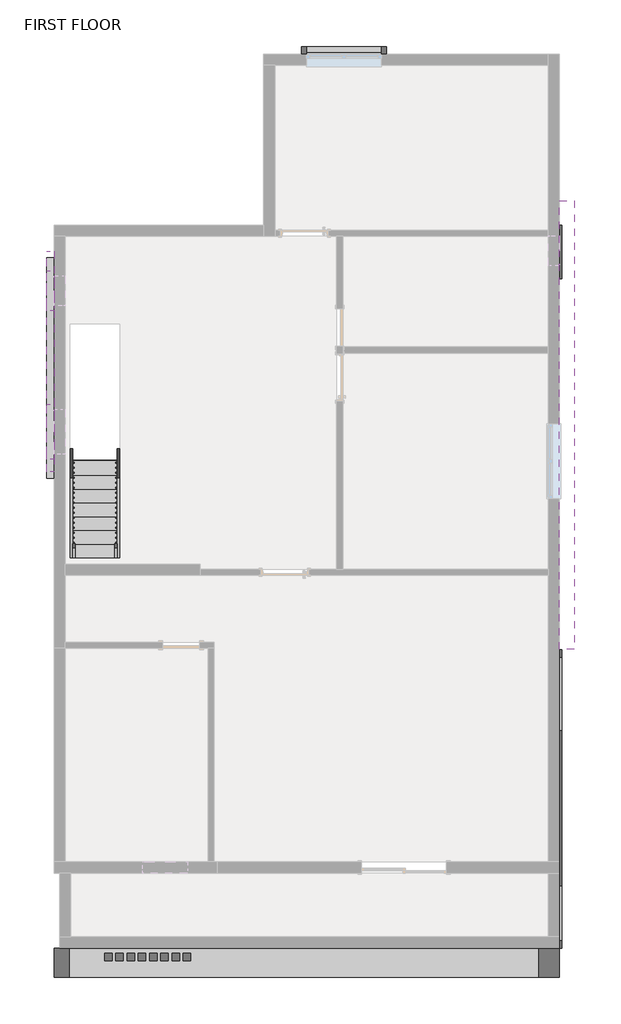
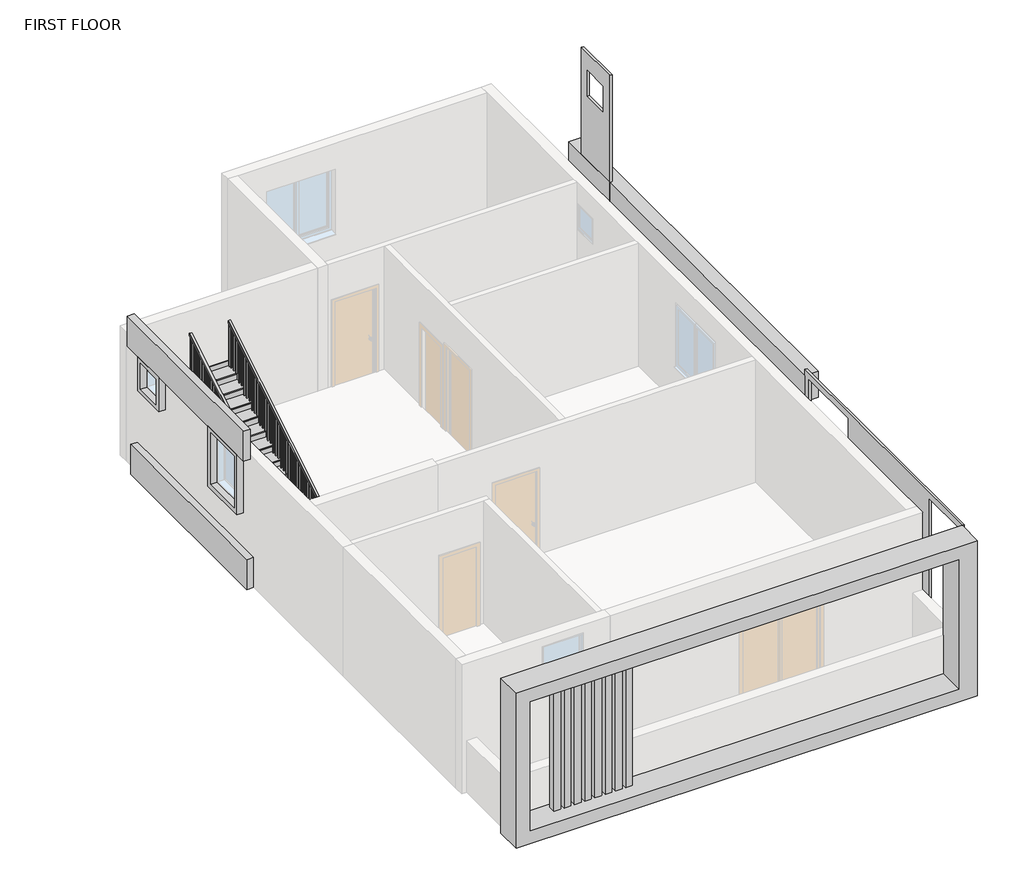
# One storey, part 2 of 2: 10 proxies, 2 members, 2 railings, 1 stair flight.
"""IFC4 building model written with IfcOpenShell, lengths in millimetres."""

from ifc_helpers import new_model, si_unit, frame, origin, place, context, project, spatial, polyline, outline, extrude, transform, mapped, element, save
from components import generic_models_11_generic_models_11_dfcfed8c, generic_models_12_generic_models_12_5399d40d, generic_models_14_generic_models_14_41b81b58, generic_models_18_generic_models_18_bc45088a, generic_models_1_generic_models_1_af82f8a7, generic_models_3_generic_models_3_c18588e6, generic_models_6_generic_models_6_b3d137af, generic_models_7_generic_models_7_06f2fd99, generic_models_8_generic_models_8_8aa07b80, stair_flight_6f7ba89f

model = new_model("IFC4")

# Units and contexts
model_context = context("Model", 3, world=origin())
ifc_project = project(units=[si_unit("LENGTHUNIT", "METRE", prefix="MILLI")], contexts=[model_context])

# Site, building, storey
site = spatial("IfcSite", under=ifc_project)
building = spatial("IfcBuilding", under=site)
storey = spatial("IfcBuildingStorey", under=building, Name="FIRST FLOOR", Elevation=3352.8)

# Proxies
placement = place(None, origin())
generic_models_11_generic_models_11_shape = generic_models_11_generic_models_11_dfcfed8c(model_context)
element("IfcBuildingElementProxy", 1, Name="Generic Models 11 : Generic Models 11", ObjectType="Generic Models 11 : Generic Models 11", at=placement, inside=storey, context=model_context, shape_type="MappedRepresentation", body=[
    mapped(generic_models_11_generic_models_11_shape, transform((0.0, 0.0, 0.0), x_axis=(1.0, 0.0, 0.0), y_axis=(0.0, 1.0, 0.0), z_axis=(0.0, 0.0, 1.0))),
])
generic_models_12_generic_models_12_shape = generic_models_12_generic_models_12_5399d40d(model_context)
element("IfcBuildingElementProxy", 2, Name="Generic Models 12 : Generic Models 12", ObjectType="Generic Models 12 : Generic Models 12", at=placement, inside=storey, context=model_context, shape_type="MappedRepresentation", body=[
    mapped(generic_models_12_generic_models_12_shape, transform((0.0, 0.0, 0.0), x_axis=(1.0, 0.0, 0.0), y_axis=(0.0, 1.0, 0.0), z_axis=(0.0, 0.0, 1.0))),
])
generic_models_14_generic_models_14_shape = generic_models_14_generic_models_14_41b81b58(model_context)
element("IfcBuildingElementProxy", 3, Name="Generic Models 14 : Generic Models 14", ObjectType="Generic Models 14 : Generic Models 14", at=placement, inside=storey, context=model_context, shape_type="MappedRepresentation", body=[
    mapped(generic_models_14_generic_models_14_shape, transform((0.0, 0.0, 0.0), x_axis=(1.0, 0.0, 0.0), y_axis=(0.0, 1.0, 0.0), z_axis=(0.0, 0.0, 1.0))),
])
element("IfcBuildingElementProxy", 4, Name="Generic Models 15 : Generic Models 14", ObjectType="Generic Models 15 : Generic Models 14", at=placement, inside=storey, context=model_context, shape_type="MappedRepresentation", body=[
    mapped(generic_models_14_generic_models_14_shape, transform((0.0, -127.0, -2946.4), x_axis=(1.0, 0.0, 0.0), y_axis=(0.0, 1.0, 0.0), z_axis=(0.0, 0.0, 1.0))),
])
generic_models_18_generic_models_18_shape = generic_models_18_generic_models_18_bc45088a(model_context)
element("IfcBuildingElementProxy", 5, Name="Generic Models 19 : Generic Models 18", ObjectType="Generic Models 19 : Generic Models 18", at=placement, inside=storey, context=model_context, shape_type="MappedRepresentation", body=[
    mapped(generic_models_18_generic_models_18_shape, transform((-152.4, 0.0, -3048.0), x_axis=(1.0, 0.0, 0.0), y_axis=(0.0, 1.0, 0.0), z_axis=(0.0, 0.0, 1.0))),
])
generic_models_1_generic_models_1_shape = generic_models_1_generic_models_1_af82f8a7(model_context)
element("IfcBuildingElementProxy", 6, Name="Generic Models 2 : Generic Models 1", ObjectType="Generic Models 2 : Generic Models 1", at=placement, inside=storey, context=model_context, shape_type="MappedRepresentation", body=[
    mapped(generic_models_1_generic_models_1_shape, transform((0.0, 0.0, 3200.4), x_axis=(1.0, 0.0, 0.0), y_axis=(0.0, 1.0, 0.0), z_axis=(0.0, 0.0, 1.0))),
])
generic_models_3_generic_models_3_shape = generic_models_3_generic_models_3_c18588e6(model_context)
element("IfcBuildingElementProxy", 7, Name="Generic Models 3 : Generic Models 3", ObjectType="Generic Models 3 : Generic Models 3", at=placement, inside=storey, context=model_context, shape_type="MappedRepresentation", body=[
    mapped(generic_models_3_generic_models_3_shape, transform((0.0, 0.0, 0.0), x_axis=(1.0, 0.0, 0.0), y_axis=(0.0, 1.0, 0.0), z_axis=(0.0, 0.0, 1.0))),
])
generic_models_6_generic_models_6_shape = generic_models_6_generic_models_6_b3d137af(model_context)
element("IfcBuildingElementProxy", 8, Name="Generic Models 6 : Generic Models 6", ObjectType="Generic Models 6 : Generic Models 6", at=placement, inside=storey, context=model_context, shape_type="MappedRepresentation", body=[
    mapped(generic_models_6_generic_models_6_shape, transform((0.0, 0.0, 0.0), x_axis=(1.0, 0.0, 0.0), y_axis=(0.0, 1.0, 0.0), z_axis=(0.0, 0.0, 1.0))),
])
generic_models_7_generic_models_7_shape = generic_models_7_generic_models_7_06f2fd99(model_context)
element("IfcBuildingElementProxy", 9, Name="Generic Models 7 : Generic Models 7", ObjectType="Generic Models 7 : Generic Models 7", at=placement, inside=storey, context=model_context, shape_type="MappedRepresentation", body=[
    mapped(generic_models_7_generic_models_7_shape, transform((0.0, 0.0, 0.0), x_axis=(1.0, 0.0, 0.0), y_axis=(0.0, 1.0, 0.0), z_axis=(0.0, 0.0, 1.0))),
])
generic_models_8_generic_models_8_shape = generic_models_8_generic_models_8_8aa07b80(model_context)
element("IfcBuildingElementProxy", 10, Name="Generic Models 8 : Generic Models 8", ObjectType="Generic Models 8 : Generic Models 8", at=placement, inside=storey, context=model_context, shape_type="MappedRepresentation", body=[
    mapped(generic_models_8_generic_models_8_shape, transform((0.0, 0.0, 0.0), x_axis=(1.0, 0.0, 0.0), y_axis=(0.0, 1.0, 0.0), z_axis=(0.0, 0.0, 1.0))),
])

# Members
element("IfcMember", 11, ObjectType="Stringer - 2\" Width", at=placement, inside=storey, context=model_context, shape_type="SweptSolid", body=[
    extrude(outline(polyline([(2020.7325341, 3352.8), (2020.7325341, 3564.914512), (6770.5325341, 6443.5811786), (6770.5325341, 6087.1724171), (2258.8180459, 3352.8), (2020.7325341, 3352.8)])), frame((-5772.3875748, 0.0, 0.0), z_axis=(1.0, 0.0, 0.0), x_axis=(0.0, 1.0, 0.0)), (0.0, 0.0, 1.0), 50.8),
])
element("IfcMember", 12, ObjectType="Stringer - 2\" Width", at=placement, inside=storey, context=model_context, shape_type="SweptSolid", body=[
    extrude(outline(polyline([(2020.7325341, 3352.8), (2020.7325341, 3564.914512), (6770.5325341, 6443.5811786), (6770.5325341, 6087.1724171), (2258.8180459, 3352.8), (2020.7325341, 3352.8)])), frame((-4807.1875748, 0.0, 0.0), z_axis=(1.0, 0.0, 0.0), x_axis=(0.0, 1.0, 0.0)), (0.0, 0.0, 1.0), 50.8),
])

# Railings
element("IfcRailing", 13, ObjectType="Handrail - Rectangular", at=placement, inside=storey, context=model_context, shape_type="SweptSolid", body=[
    extrude(outline(polyline([(2020.7325341, 4377.1318731), (2020.7325341, 4436.5333333), (6770.5325341, 7315.2), (6770.5325341, 7255.7985397), (2020.7325341, 4377.1318731)])), frame((-4857.9875748, 0.0, 0.0), z_axis=(1.0, 0.0, 0.0), x_axis=(0.0, 1.0, 0.0)), (0.0, 0.0, 1.0), 50.8),
    extrude(outline(polyline([(6684.8075341, 7203.8439943), (6703.8575341, 7215.3894488), (6703.8575341, 6231.4666667), (6684.8075341, 6231.4666667), (6684.8075341, 7203.8439943)])), frame((-4842.1125748, 0.0, 0.0), z_axis=(1.0, 0.0, 0.0), x_axis=(0.0, 1.0, 0.0)), (0.0, 0.0, 1.0), 19.05),
    extrude(outline(polyline([(6583.2075341, 7142.2682367), (6602.2575341, 7153.8136913), (6602.2575341, 6231.4666667), (6583.2075341, 6231.4666667), (6583.2075341, 7142.2682367)])), frame((-4842.1125748, 0.0, 0.0), z_axis=(1.0, 0.0, 0.0), x_axis=(0.0, 1.0, 0.0)), (0.0, 0.0, 1.0), 19.05),
    extrude(outline(polyline([(6481.6075341, 7080.6924791), (6500.6575341, 7092.2379337), (6500.6575341, 6231.4666667), (6481.6075341, 6231.4666667), (6481.6075341, 7080.6924791)])), frame((-4842.1125748, 0.0, 0.0), z_axis=(1.0, 0.0, 0.0), x_axis=(0.0, 1.0, 0.0)), (0.0, 0.0, 1.0), 19.05),
    extrude(outline(polyline([(6380.0075341, 7019.1167216), (6399.0575341, 7030.6621761), (6399.0575341, 6062.1333333), (6380.0075341, 6062.1333333), (6380.0075341, 7019.1167216)])), frame((-4842.1125748, 0.0, 0.0), z_axis=(1.0, 0.0, 0.0), x_axis=(0.0, 1.0, 0.0)), (0.0, 0.0, 1.0), 19.05),
    extrude(outline(polyline([(6278.4075341, 6957.540964), (6297.4575341, 6969.0864185), (6297.4575341, 6062.1333333), (6278.4075341, 6062.1333333), (6278.4075341, 6957.540964)])), frame((-4842.1125748, 0.0, 0.0), z_axis=(1.0, 0.0, 0.0), x_axis=(0.0, 1.0, 0.0)), (0.0, 0.0, 1.0), 19.05),
    extrude(outline(polyline([(6176.8075341, 6895.9652064), (6195.8575341, 6907.510661), (6195.8575341, 5892.8), (6176.8075341, 5892.8), (6176.8075341, 6895.9652064)])), frame((-4842.1125748, 0.0, 0.0), z_axis=(1.0, 0.0, 0.0), x_axis=(0.0, 1.0, 0.0)), (0.0, 0.0, 1.0), 19.05),
    extrude(outline(polyline([(6075.2075341, 6834.3894488), (6094.2575341, 6845.9349034), (6094.2575341, 5892.8), (6075.2075341, 5892.8), (6075.2075341, 6834.3894488)])), frame((-4842.1125748, 0.0, 0.0), z_axis=(1.0, 0.0, 0.0), x_axis=(0.0, 1.0, 0.0)), (0.0, 0.0, 1.0), 19.05),
    extrude(outline(polyline([(5973.6075341, 6772.8136913), (5992.6575341, 6784.3591458), (5992.6575341, 5892.8), (5973.6075341, 5892.8), (5973.6075341, 6772.8136913)])), frame((-4842.1125748, 0.0, 0.0), z_axis=(1.0, 0.0, 0.0), x_axis=(0.0, 1.0, 0.0)), (0.0, 0.0, 1.0), 19.05),
    extrude(outline(polyline([(5872.0075341, 6711.2379337), (5891.0575341, 6722.7833882), (5891.0575341, 5723.4666667), (5872.0075341, 5723.4666667), (5872.0075341, 6711.2379337)])), frame((-4842.1125748, 0.0, 0.0), z_axis=(1.0, 0.0, 0.0), x_axis=(0.0, 1.0, 0.0)), (0.0, 0.0, 1.0), 19.05),
    extrude(outline(polyline([(5770.4075341, 6649.6621761), (5789.4575341, 6661.2076307), (5789.4575341, 5723.4666667), (5770.4075341, 5723.4666667), (5770.4075341, 6649.6621761)])), frame((-4842.1125748, 0.0, 0.0), z_axis=(1.0, 0.0, 0.0), x_axis=(0.0, 1.0, 0.0)), (0.0, 0.0, 1.0), 19.05),
    extrude(outline(polyline([(5668.8075341, 6588.0864185), (5687.8575341, 6599.6318731), (5687.8575341, 5723.4666667), (5668.8075341, 5723.4666667), (5668.8075341, 6588.0864185)])), frame((-4842.1125748, 0.0, 0.0), z_axis=(1.0, 0.0, 0.0), x_axis=(0.0, 1.0, 0.0)), (0.0, 0.0, 1.0), 19.05),
    extrude(outline(polyline([(5567.2075341, 6526.510661), (5586.2575341, 6538.0561155), (5586.2575341, 5554.1333333), (5567.2075341, 5554.1333333), (5567.2075341, 6526.510661)])), frame((-4842.1125748, 0.0, 0.0), z_axis=(1.0, 0.0, 0.0), x_axis=(0.0, 1.0, 0.0)), (0.0, 0.0, 1.0), 19.05),
    extrude(outline(polyline([(5465.6075341, 6464.9349034), (5484.6575341, 6476.4803579), (5484.6575341, 5554.1333333), (5465.6075341, 5554.1333333), (5465.6075341, 6464.9349034)])), frame((-4842.1125748, 0.0, 0.0), z_axis=(1.0, 0.0, 0.0), x_axis=(0.0, 1.0, 0.0)), (0.0, 0.0, 1.0), 19.05),
    extrude(outline(polyline([(5364.0075341, 6403.3591458), (5383.0575341, 6414.9046004), (5383.0575341, 5554.1333333), (5364.0075341, 5554.1333333), (5364.0075341, 6403.3591458)])), frame((-4842.1125748, 0.0, 0.0), z_axis=(1.0, 0.0, 0.0), x_axis=(0.0, 1.0, 0.0)), (0.0, 0.0, 1.0), 19.05),
    extrude(outline(polyline([(5262.4075341, 6341.7833882), (5281.4575341, 6353.3288428), (5281.4575341, 5384.8), (5262.4075341, 5384.8), (5262.4075341, 6341.7833882)])), frame((-4842.1125748, 0.0, 0.0), z_axis=(1.0, 0.0, 0.0), x_axis=(0.0, 1.0, 0.0)), (0.0, 0.0, 1.0), 19.05),
    extrude(outline(polyline([(5160.8075341, 6280.2076307), (5179.8575341, 6291.7530852), (5179.8575341, 5384.8), (5160.8075341, 5384.8), (5160.8075341, 6280.2076307)])), frame((-4842.1125748, 0.0, 0.0), z_axis=(1.0, 0.0, 0.0), x_axis=(0.0, 1.0, 0.0)), (0.0, 0.0, 1.0), 19.05),
    extrude(outline(polyline([(5059.2075341, 6218.6318731), (5078.2575341, 6230.1773276), (5078.2575341, 5215.4666667), (5059.2075341, 5215.4666667), (5059.2075341, 6218.6318731)])), frame((-4842.1125748, 0.0, 0.0), z_axis=(1.0, 0.0, 0.0), x_axis=(0.0, 1.0, 0.0)), (0.0, 0.0, 1.0), 19.05),
    extrude(outline(polyline([(4957.6075341, 6157.0561155), (4976.6575341, 6168.60157), (4976.6575341, 5215.4666667), (4957.6075341, 5215.4666667), (4957.6075341, 6157.0561155)])), frame((-4842.1125748, 0.0, 0.0), z_axis=(1.0, 0.0, 0.0), x_axis=(0.0, 1.0, 0.0)), (0.0, 0.0, 1.0), 19.05),
    extrude(outline(polyline([(4856.0075341, 6095.4803579), (4875.0575341, 6107.0258125), (4875.0575341, 5215.4666667), (4856.0075341, 5215.4666667), (4856.0075341, 6095.4803579)])), frame((-4842.1125748, 0.0, 0.0), z_axis=(1.0, 0.0, 0.0), x_axis=(0.0, 1.0, 0.0)), (0.0, 0.0, 1.0), 19.05),
    extrude(outline(polyline([(4754.4075341, 6033.9046004), (4773.4575341, 6045.4500549), (4773.4575341, 5046.1333333), (4754.4075341, 5046.1333333), (4754.4075341, 6033.9046004)])), frame((-4842.1125748, 0.0, 0.0), z_axis=(1.0, 0.0, 0.0), x_axis=(0.0, 1.0, 0.0)), (0.0, 0.0, 1.0), 19.05),
    extrude(outline(polyline([(4652.8075341, 5972.3288428), (4671.8575341, 5983.8742973), (4671.8575341, 5046.1333333), (4652.8075341, 5046.1333333), (4652.8075341, 5972.3288428)])), frame((-4842.1125748, 0.0, 0.0), z_axis=(1.0, 0.0, 0.0), x_axis=(0.0, 1.0, 0.0)), (0.0, 0.0, 1.0), 19.05),
    extrude(outline(polyline([(4551.2075341, 5910.7530852), (4570.2575341, 5922.2985397), (4570.2575341, 5046.1333333), (4551.2075341, 5046.1333333), (4551.2075341, 5910.7530852)])), frame((-4842.1125748, 0.0, 0.0), z_axis=(1.0, 0.0, 0.0), x_axis=(0.0, 1.0, 0.0)), (0.0, 0.0, 1.0), 19.05),
    extrude(outline(polyline([(4449.6075341, 5849.1773276), (4468.6575341, 5860.7227822), (4468.6575341, 4876.8), (4449.6075341, 4876.8), (4449.6075341, 5849.1773276)])), frame((-4842.1125748, 0.0, 0.0), z_axis=(1.0, 0.0, 0.0), x_axis=(0.0, 1.0, 0.0)), (0.0, 0.0, 1.0), 19.05),
    extrude(outline(polyline([(4348.0075341, 5787.60157), (4367.0575341, 5799.1470246), (4367.0575341, 4876.8), (4348.0075341, 4876.8), (4348.0075341, 5787.60157)])), frame((-4842.1125748, 0.0, 0.0), z_axis=(1.0, 0.0, 0.0), x_axis=(0.0, 1.0, 0.0)), (0.0, 0.0, 1.0), 19.05),
    extrude(outline(polyline([(4246.4075341, 5726.0258125), (4265.4575341, 5737.571267), (4265.4575341, 4876.8), (4246.4075341, 4876.8), (4246.4075341, 5726.0258125)])), frame((-4842.1125748, 0.0, 0.0), z_axis=(1.0, 0.0, 0.0), x_axis=(0.0, 1.0, 0.0)), (0.0, 0.0, 1.0), 19.05),
    extrude(outline(polyline([(4144.8075341, 5664.4500549), (4163.8575341, 5675.9955094), (4163.8575341, 4707.4666667), (4144.8075341, 4707.4666667), (4144.8075341, 5664.4500549)])), frame((-4842.1125748, 0.0, 0.0), z_axis=(1.0, 0.0, 0.0), x_axis=(0.0, 1.0, 0.0)), (0.0, 0.0, 1.0), 19.05),
    extrude(outline(polyline([(4043.2075341, 5602.8742973), (4062.2575341, 5614.4197519), (4062.2575341, 4707.4666667), (4043.2075341, 4707.4666667), (4043.2075341, 5602.8742973)])), frame((-4842.1125748, 0.0, 0.0), z_axis=(1.0, 0.0, 0.0), x_axis=(0.0, 1.0, 0.0)), (0.0, 0.0, 1.0), 19.05),
    extrude(outline(polyline([(3941.6075341, 5541.2985397), (3960.6575341, 5552.8439943), (3960.6575341, 4538.1333333), (3941.6075341, 4538.1333333), (3941.6075341, 5541.2985397)])), frame((-4842.1125748, 0.0, 0.0), z_axis=(1.0, 0.0, 0.0), x_axis=(0.0, 1.0, 0.0)), (0.0, 0.0, 1.0), 19.05),
    extrude(outline(polyline([(3840.0075341, 5479.7227822), (3859.0575341, 5491.2682367), (3859.0575341, 4538.1333333), (3840.0075341, 4538.1333333), (3840.0075341, 5479.7227822)])), frame((-4842.1125748, 0.0, 0.0), z_axis=(1.0, 0.0, 0.0), x_axis=(0.0, 1.0, 0.0)), (0.0, 0.0, 1.0), 19.05),
    extrude(outline(polyline([(3738.4075341, 5418.1470246), (3757.4575341, 5429.6924791), (3757.4575341, 4538.1333333), (3738.4075341, 4538.1333333), (3738.4075341, 5418.1470246)])), frame((-4842.1125748, 0.0, 0.0), z_axis=(1.0, 0.0, 0.0), x_axis=(0.0, 1.0, 0.0)), (0.0, 0.0, 1.0), 19.05),
    extrude(outline(polyline([(3636.8075341, 5356.571267), (3655.8575341, 5368.1167216), (3655.8575341, 4368.8), (3636.8075341, 4368.8), (3636.8075341, 5356.571267)])), frame((-4842.1125748, 0.0, 0.0), z_axis=(1.0, 0.0, 0.0), x_axis=(0.0, 1.0, 0.0)), (0.0, 0.0, 1.0), 19.05),
    extrude(outline(polyline([(3535.2075341, 5294.9955094), (3554.2575341, 5306.540964), (3554.2575341, 4368.8), (3535.2075341, 4368.8), (3535.2075341, 5294.9955094)])), frame((-4842.1125748, 0.0, 0.0), z_axis=(1.0, 0.0, 0.0), x_axis=(0.0, 1.0, 0.0)), (0.0, 0.0, 1.0), 19.05),
    extrude(outline(polyline([(3433.6075341, 5233.4197519), (3452.6575341, 5244.9652064), (3452.6575341, 4368.8), (3433.6075341, 4368.8), (3433.6075341, 5233.4197519)])), frame((-4842.1125748, 0.0, 0.0), z_axis=(1.0, 0.0, 0.0), x_axis=(0.0, 1.0, 0.0)), (0.0, 0.0, 1.0), 19.05),
    extrude(outline(polyline([(3332.0075341, 5171.8439943), (3351.0575341, 5183.3894488), (3351.0575341, 4199.4666667), (3332.0075341, 4199.4666667), (3332.0075341, 5171.8439943)])), frame((-4842.1125748, 0.0, 0.0), z_axis=(1.0, 0.0, 0.0), x_axis=(0.0, 1.0, 0.0)), (0.0, 0.0, 1.0), 19.05),
    extrude(outline(polyline([(3230.4075341, 5110.2682367), (3249.4575341, 5121.8136913), (3249.4575341, 4199.4666667), (3230.4075341, 4199.4666667), (3230.4075341, 5110.2682367)])), frame((-4842.1125748, 0.0, 0.0), z_axis=(1.0, 0.0, 0.0), x_axis=(0.0, 1.0, 0.0)), (0.0, 0.0, 1.0), 19.05),
    extrude(outline(polyline([(3128.8075341, 5048.6924791), (3147.8575341, 5060.2379337), (3147.8575341, 4199.4666667), (3128.8075341, 4199.4666667), (3128.8075341, 5048.6924791)])), frame((-4842.1125748, 0.0, 0.0), z_axis=(1.0, 0.0, 0.0), x_axis=(0.0, 1.0, 0.0)), (0.0, 0.0, 1.0), 19.05),
    extrude(outline(polyline([(3027.2075341, 4987.1167216), (3046.2575341, 4998.6621761), (3046.2575341, 4030.1333333), (3027.2075341, 4030.1333333), (3027.2075341, 4987.1167216)])), frame((-4842.1125748, 0.0, 0.0), z_axis=(1.0, 0.0, 0.0), x_axis=(0.0, 1.0, 0.0)), (0.0, 0.0, 1.0), 19.05),
    extrude(outline(polyline([(2925.6075341, 4925.540964), (2944.6575341, 4937.0864185), (2944.6575341, 4030.1333333), (2925.6075341, 4030.1333333), (2925.6075341, 4925.540964)])), frame((-4842.1125748, 0.0, 0.0), z_axis=(1.0, 0.0, 0.0), x_axis=(0.0, 1.0, 0.0)), (0.0, 0.0, 1.0), 19.05),
    extrude(outline(polyline([(2824.0075341, 4863.9652064), (2843.0575341, 4875.510661), (2843.0575341, 3860.8), (2824.0075341, 3860.8), (2824.0075341, 4863.9652064)])), frame((-4842.1125748, 0.0, 0.0), z_axis=(1.0, 0.0, 0.0), x_axis=(0.0, 1.0, 0.0)), (0.0, 0.0, 1.0), 19.05),
    extrude(outline(polyline([(2722.4075341, 4802.3894488), (2741.4575341, 4813.9349034), (2741.4575341, 3860.8), (2722.4075341, 3860.8), (2722.4075341, 4802.3894488)])), frame((-4842.1125748, 0.0, 0.0), z_axis=(1.0, 0.0, 0.0), x_axis=(0.0, 1.0, 0.0)), (0.0, 0.0, 1.0), 19.05),
    extrude(outline(polyline([(2620.8075341, 4740.8136913), (2639.8575341, 4752.3591458), (2639.8575341, 3860.8), (2620.8075341, 3860.8), (2620.8075341, 4740.8136913)])), frame((-4842.1125748, 0.0, 0.0), z_axis=(1.0, 0.0, 0.0), x_axis=(0.0, 1.0, 0.0)), (0.0, 0.0, 1.0), 19.05),
    extrude(outline(polyline([(2519.2075341, 4679.2379337), (2538.2575341, 4690.7833882), (2538.2575341, 3691.4666667), (2519.2075341, 3691.4666667), (2519.2075341, 4679.2379337)])), frame((-4842.1125748, 0.0, 0.0), z_axis=(1.0, 0.0, 0.0), x_axis=(0.0, 1.0, 0.0)), (0.0, 0.0, 1.0), 19.05),
    extrude(outline(polyline([(2417.6075341, 4617.6621761), (2436.6575341, 4629.2076307), (2436.6575341, 3691.4666667), (2417.6075341, 3691.4666667), (2417.6075341, 4617.6621761)])), frame((-4842.1125748, 0.0, 0.0), z_axis=(1.0, 0.0, 0.0), x_axis=(0.0, 1.0, 0.0)), (0.0, 0.0, 1.0), 19.05),
    extrude(outline(polyline([(2316.0075341, 4556.0864185), (2335.0575341, 4567.6318731), (2335.0575341, 3691.4666667), (2316.0075341, 3691.4666667), (2316.0075341, 4556.0864185)])), frame((-4842.1125748, 0.0, 0.0), z_axis=(1.0, 0.0, 0.0), x_axis=(0.0, 1.0, 0.0)), (0.0, 0.0, 1.0), 19.05),
    extrude(outline(polyline([(2214.4075341, 4494.510661), (2233.4575341, 4506.0561155), (2233.4575341, 3522.1333333), (2214.4075341, 3522.1333333), (2214.4075341, 4494.510661)])), frame((-4842.1125748, 0.0, 0.0), z_axis=(1.0, 0.0, 0.0), x_axis=(0.0, 1.0, 0.0)), (0.0, 0.0, 1.0), 19.05),
    extrude(outline(polyline([(2112.8075341, 4432.9349034), (2131.8575341, 4444.4803579), (2131.8575341, 3522.1333333), (2112.8075341, 3522.1333333), (2112.8075341, 4432.9349034)])), frame((-4842.1125748, 0.0, 0.0), z_axis=(1.0, 0.0, 0.0), x_axis=(0.0, 1.0, 0.0)), (0.0, 0.0, 1.0), 19.05),
    extrude(outline(polyline([(6751.4825341, 7244.2530852), (6770.5325341, 7255.7985397), (6770.5325341, 6231.4666667), (6751.4825341, 6231.4666667), (6751.4825341, 7244.2530852)])), frame((-4842.1125748, 0.0, 0.0), z_axis=(1.0, 0.0, 0.0), x_axis=(0.0, 1.0, 0.0)), (0.0, 0.0, 1.0), 19.05),
    extrude(outline(polyline([(2020.7325341, 4377.1318731), (2039.7825341, 4388.6773276), (2039.7825341, 3522.1333333), (2020.7325341, 3522.1333333), (2020.7325341, 4377.1318731)])), frame((-4842.1125748, 0.0, 0.0), z_axis=(1.0, 0.0, 0.0), x_axis=(0.0, 1.0, 0.0)), (0.0, 0.0, 1.0), 19.05),
])
element("IfcRailing", 14, ObjectType="Handrail - Rectangular", at=placement, inside=storey, context=model_context, shape_type="SweptSolid", body=[
    extrude(outline(polyline([(2020.7325341, 4377.1318731), (2020.7325341, 4436.5333333), (6770.5325341, 7315.2), (6770.5325341, 7255.7985397), (2020.7325341, 4377.1318731)])), frame((-5721.5875748, 0.0, 0.0), z_axis=(1.0, 0.0, 0.0), x_axis=(0.0, 1.0, 0.0)), (0.0, 0.0, 1.0), 50.8),
    extrude(outline(polyline([(6703.8575341, 7215.3894488), (6703.8575341, 6231.4666667), (6684.8075341, 6231.4666667), (6684.8075341, 7203.8439943), (6703.8575341, 7215.3894488)])), frame((-5705.7125748, 0.0, 0.0), z_axis=(1.0, 0.0, 0.0), x_axis=(0.0, 1.0, 0.0)), (0.0, 0.0, 1.0), 19.05),
    extrude(outline(polyline([(6602.2575341, 7153.8136913), (6602.2575341, 6231.4666667), (6583.2075341, 6231.4666667), (6583.2075341, 7142.2682367), (6602.2575341, 7153.8136913)])), frame((-5705.7125748, 0.0, 0.0), z_axis=(1.0, 0.0, 0.0), x_axis=(0.0, 1.0, 0.0)), (0.0, 0.0, 1.0), 19.05),
    extrude(outline(polyline([(6500.6575341, 7092.2379337), (6500.6575341, 6231.4666667), (6481.6075341, 6231.4666667), (6481.6075341, 7080.6924791), (6500.6575341, 7092.2379337)])), frame((-5705.7125748, 0.0, 0.0), z_axis=(1.0, 0.0, 0.0), x_axis=(0.0, 1.0, 0.0)), (0.0, 0.0, 1.0), 19.05),
    extrude(outline(polyline([(6399.0575341, 7030.6621761), (6399.0575341, 6062.1333333), (6380.0075341, 6062.1333333), (6380.0075341, 7019.1167216), (6399.0575341, 7030.6621761)])), frame((-5705.7125748, 0.0, 0.0), z_axis=(1.0, 0.0, 0.0), x_axis=(0.0, 1.0, 0.0)), (0.0, 0.0, 1.0), 19.05),
    extrude(outline(polyline([(6297.4575341, 6969.0864185), (6297.4575341, 6062.1333333), (6278.4075341, 6062.1333333), (6278.4075341, 6957.540964), (6297.4575341, 6969.0864185)])), frame((-5705.7125748, 0.0, 0.0), z_axis=(1.0, 0.0, 0.0), x_axis=(0.0, 1.0, 0.0)), (0.0, 0.0, 1.0), 19.05),
    extrude(outline(polyline([(6195.8575341, 6907.510661), (6195.8575341, 5892.8), (6176.8075341, 5892.8), (6176.8075341, 6895.9652064), (6195.8575341, 6907.510661)])), frame((-5705.7125748, 0.0, 0.0), z_axis=(1.0, 0.0, 0.0), x_axis=(0.0, 1.0, 0.0)), (0.0, 0.0, 1.0), 19.05),
    extrude(outline(polyline([(6094.2575341, 6845.9349034), (6094.2575341, 5892.8), (6075.2075341, 5892.8), (6075.2075341, 6834.3894488), (6094.2575341, 6845.9349034)])), frame((-5705.7125748, 0.0, 0.0), z_axis=(1.0, 0.0, 0.0), x_axis=(0.0, 1.0, 0.0)), (0.0, 0.0, 1.0), 19.05),
    extrude(outline(polyline([(5992.6575341, 6784.3591458), (5992.6575341, 5892.8), (5973.6075341, 5892.8), (5973.6075341, 6772.8136913), (5992.6575341, 6784.3591458)])), frame((-5705.7125748, 0.0, 0.0), z_axis=(1.0, 0.0, 0.0), x_axis=(0.0, 1.0, 0.0)), (0.0, 0.0, 1.0), 19.05),
    extrude(outline(polyline([(5891.0575341, 6722.7833882), (5891.0575341, 5723.4666667), (5872.0075341, 5723.4666667), (5872.0075341, 6711.2379337), (5891.0575341, 6722.7833882)])), frame((-5705.7125748, 0.0, 0.0), z_axis=(1.0, 0.0, 0.0), x_axis=(0.0, 1.0, 0.0)), (0.0, 0.0, 1.0), 19.05),
    extrude(outline(polyline([(5789.4575341, 6661.2076307), (5789.4575341, 5723.4666667), (5770.4075341, 5723.4666667), (5770.4075341, 6649.6621761), (5789.4575341, 6661.2076307)])), frame((-5705.7125748, 0.0, 0.0), z_axis=(1.0, 0.0, 0.0), x_axis=(0.0, 1.0, 0.0)), (0.0, 0.0, 1.0), 19.05),
    extrude(outline(polyline([(5687.8575341, 6599.6318731), (5687.8575341, 5723.4666667), (5668.8075341, 5723.4666667), (5668.8075341, 6588.0864185), (5687.8575341, 6599.6318731)])), frame((-5705.7125748, 0.0, 0.0), z_axis=(1.0, 0.0, 0.0), x_axis=(0.0, 1.0, 0.0)), (0.0, 0.0, 1.0), 19.05),
    extrude(outline(polyline([(5586.2575341, 6538.0561155), (5586.2575341, 5554.1333333), (5567.2075341, 5554.1333333), (5567.2075341, 6526.510661), (5586.2575341, 6538.0561155)])), frame((-5705.7125748, 0.0, 0.0), z_axis=(1.0, 0.0, 0.0), x_axis=(0.0, 1.0, 0.0)), (0.0, 0.0, 1.0), 19.05),
    extrude(outline(polyline([(5484.6575341, 6476.4803579), (5484.6575341, 5554.1333333), (5465.6075341, 5554.1333333), (5465.6075341, 6464.9349034), (5484.6575341, 6476.4803579)])), frame((-5705.7125748, 0.0, 0.0), z_axis=(1.0, 0.0, 0.0), x_axis=(0.0, 1.0, 0.0)), (0.0, 0.0, 1.0), 19.05),
    extrude(outline(polyline([(5383.0575341, 6414.9046004), (5383.0575341, 5554.1333333), (5364.0075341, 5554.1333333), (5364.0075341, 6403.3591458), (5383.0575341, 6414.9046004)])), frame((-5705.7125748, 0.0, 0.0), z_axis=(1.0, 0.0, 0.0), x_axis=(0.0, 1.0, 0.0)), (0.0, 0.0, 1.0), 19.05),
    extrude(outline(polyline([(5281.4575341, 6353.3288428), (5281.4575341, 5384.8), (5262.4075341, 5384.8), (5262.4075341, 6341.7833882), (5281.4575341, 6353.3288428)])), frame((-5705.7125748, 0.0, 0.0), z_axis=(1.0, 0.0, 0.0), x_axis=(0.0, 1.0, 0.0)), (0.0, 0.0, 1.0), 19.05),
    extrude(outline(polyline([(5179.8575341, 6291.7530852), (5179.8575341, 5384.8), (5160.8075341, 5384.8), (5160.8075341, 6280.2076307), (5179.8575341, 6291.7530852)])), frame((-5705.7125748, 0.0, 0.0), z_axis=(1.0, 0.0, 0.0), x_axis=(0.0, 1.0, 0.0)), (0.0, 0.0, 1.0), 19.05),
    extrude(outline(polyline([(5078.2575341, 6230.1773276), (5078.2575341, 5215.4666667), (5059.2075341, 5215.4666667), (5059.2075341, 6218.6318731), (5078.2575341, 6230.1773276)])), frame((-5705.7125748, 0.0, 0.0), z_axis=(1.0, 0.0, 0.0), x_axis=(0.0, 1.0, 0.0)), (0.0, 0.0, 1.0), 19.05),
    extrude(outline(polyline([(4976.6575341, 6168.60157), (4976.6575341, 5215.4666667), (4957.6075341, 5215.4666667), (4957.6075341, 6157.0561155), (4976.6575341, 6168.60157)])), frame((-5705.7125748, 0.0, 0.0), z_axis=(1.0, 0.0, 0.0), x_axis=(0.0, 1.0, 0.0)), (0.0, 0.0, 1.0), 19.05),
    extrude(outline(polyline([(4875.0575341, 6107.0258125), (4875.0575341, 5215.4666667), (4856.0075341, 5215.4666667), (4856.0075341, 6095.4803579), (4875.0575341, 6107.0258125)])), frame((-5705.7125748, 0.0, 0.0), z_axis=(1.0, 0.0, 0.0), x_axis=(0.0, 1.0, 0.0)), (0.0, 0.0, 1.0), 19.05),
    extrude(outline(polyline([(4773.4575341, 6045.4500549), (4773.4575341, 5046.1333333), (4754.4075341, 5046.1333333), (4754.4075341, 6033.9046004), (4773.4575341, 6045.4500549)])), frame((-5705.7125748, 0.0, 0.0), z_axis=(1.0, 0.0, 0.0), x_axis=(0.0, 1.0, 0.0)), (0.0, 0.0, 1.0), 19.05),
    extrude(outline(polyline([(4671.8575341, 5983.8742973), (4671.8575341, 5046.1333333), (4652.8075341, 5046.1333333), (4652.8075341, 5972.3288428), (4671.8575341, 5983.8742973)])), frame((-5705.7125748, 0.0, 0.0), z_axis=(1.0, 0.0, 0.0), x_axis=(0.0, 1.0, 0.0)), (0.0, 0.0, 1.0), 19.05),
    extrude(outline(polyline([(4570.2575341, 5922.2985397), (4570.2575341, 5046.1333333), (4551.2075341, 5046.1333333), (4551.2075341, 5910.7530852), (4570.2575341, 5922.2985397)])), frame((-5705.7125748, 0.0, 0.0), z_axis=(1.0, 0.0, 0.0), x_axis=(0.0, 1.0, 0.0)), (0.0, 0.0, 1.0), 19.05),
    extrude(outline(polyline([(4468.6575341, 5860.7227822), (4468.6575341, 4876.8), (4449.6075341, 4876.8), (4449.6075341, 5849.1773276), (4468.6575341, 5860.7227822)])), frame((-5705.7125748, 0.0, 0.0), z_axis=(1.0, 0.0, 0.0), x_axis=(0.0, 1.0, 0.0)), (0.0, 0.0, 1.0), 19.05),
    extrude(outline(polyline([(4367.0575341, 5799.1470246), (4367.0575341, 4876.8), (4348.0075341, 4876.8), (4348.0075341, 5787.60157), (4367.0575341, 5799.1470246)])), frame((-5705.7125748, 0.0, 0.0), z_axis=(1.0, 0.0, 0.0), x_axis=(0.0, 1.0, 0.0)), (0.0, 0.0, 1.0), 19.05),
    extrude(outline(polyline([(4265.4575341, 5737.571267), (4265.4575341, 4876.8), (4246.4075341, 4876.8), (4246.4075341, 5726.0258125), (4265.4575341, 5737.571267)])), frame((-5705.7125748, 0.0, 0.0), z_axis=(1.0, 0.0, 0.0), x_axis=(0.0, 1.0, 0.0)), (0.0, 0.0, 1.0), 19.05),
    extrude(outline(polyline([(4163.8575341, 5675.9955094), (4163.8575341, 4707.4666667), (4144.8075341, 4707.4666667), (4144.8075341, 5664.4500549), (4163.8575341, 5675.9955094)])), frame((-5705.7125748, 0.0, 0.0), z_axis=(1.0, 0.0, 0.0), x_axis=(0.0, 1.0, 0.0)), (0.0, 0.0, 1.0), 19.05),
    extrude(outline(polyline([(4062.2575341, 5614.4197519), (4062.2575341, 4707.4666667), (4043.2075341, 4707.4666667), (4043.2075341, 5602.8742973), (4062.2575341, 5614.4197519)])), frame((-5705.7125748, 0.0, 0.0), z_axis=(1.0, 0.0, 0.0), x_axis=(0.0, 1.0, 0.0)), (0.0, 0.0, 1.0), 19.05),
    extrude(outline(polyline([(3960.6575341, 5552.8439943), (3960.6575341, 4538.1333333), (3941.6075341, 4538.1333333), (3941.6075341, 5541.2985397), (3960.6575341, 5552.8439943)])), frame((-5705.7125748, 0.0, 0.0), z_axis=(1.0, 0.0, 0.0), x_axis=(0.0, 1.0, 0.0)), (0.0, 0.0, 1.0), 19.05),
    extrude(outline(polyline([(3859.0575341, 5491.2682367), (3859.0575341, 4538.1333333), (3840.0075341, 4538.1333333), (3840.0075341, 5479.7227822), (3859.0575341, 5491.2682367)])), frame((-5705.7125748, 0.0, 0.0), z_axis=(1.0, 0.0, 0.0), x_axis=(0.0, 1.0, 0.0)), (0.0, 0.0, 1.0), 19.05),
    extrude(outline(polyline([(3757.4575341, 5429.6924791), (3757.4575341, 4538.1333333), (3738.4075341, 4538.1333333), (3738.4075341, 5418.1470246), (3757.4575341, 5429.6924791)])), frame((-5705.7125748, 0.0, 0.0), z_axis=(1.0, 0.0, 0.0), x_axis=(0.0, 1.0, 0.0)), (0.0, 0.0, 1.0), 19.05),
    extrude(outline(polyline([(3655.8575341, 5368.1167216), (3655.8575341, 4368.8), (3636.8075341, 4368.8), (3636.8075341, 5356.571267), (3655.8575341, 5368.1167216)])), frame((-5705.7125748, 0.0, 0.0), z_axis=(1.0, 0.0, 0.0), x_axis=(0.0, 1.0, 0.0)), (0.0, 0.0, 1.0), 19.05),
    extrude(outline(polyline([(3554.2575341, 5306.540964), (3554.2575341, 4368.8), (3535.2075341, 4368.8), (3535.2075341, 5294.9955094), (3554.2575341, 5306.540964)])), frame((-5705.7125748, 0.0, 0.0), z_axis=(1.0, 0.0, 0.0), x_axis=(0.0, 1.0, 0.0)), (0.0, 0.0, 1.0), 19.05),
    extrude(outline(polyline([(3452.6575341, 5244.9652064), (3452.6575341, 4368.8), (3433.6075341, 4368.8), (3433.6075341, 5233.4197519), (3452.6575341, 5244.9652064)])), frame((-5705.7125748, 0.0, 0.0), z_axis=(1.0, 0.0, 0.0), x_axis=(0.0, 1.0, 0.0)), (0.0, 0.0, 1.0), 19.05),
    extrude(outline(polyline([(3351.0575341, 5183.3894488), (3351.0575341, 4199.4666667), (3332.0075341, 4199.4666667), (3332.0075341, 5171.8439943), (3351.0575341, 5183.3894488)])), frame((-5705.7125748, 0.0, 0.0), z_axis=(1.0, 0.0, 0.0), x_axis=(0.0, 1.0, 0.0)), (0.0, 0.0, 1.0), 19.05),
    extrude(outline(polyline([(3249.4575341, 5121.8136913), (3249.4575341, 4199.4666667), (3230.4075341, 4199.4666667), (3230.4075341, 5110.2682367), (3249.4575341, 5121.8136913)])), frame((-5705.7125748, 0.0, 0.0), z_axis=(1.0, 0.0, 0.0), x_axis=(0.0, 1.0, 0.0)), (0.0, 0.0, 1.0), 19.05),
    extrude(outline(polyline([(3147.8575341, 5060.2379337), (3147.8575341, 4199.4666667), (3128.8075341, 4199.4666667), (3128.8075341, 5048.6924791), (3147.8575341, 5060.2379337)])), frame((-5705.7125748, 0.0, 0.0), z_axis=(1.0, 0.0, 0.0), x_axis=(0.0, 1.0, 0.0)), (0.0, 0.0, 1.0), 19.05),
    extrude(outline(polyline([(3046.2575341, 4998.6621761), (3046.2575341, 4030.1333333), (3027.2075341, 4030.1333333), (3027.2075341, 4987.1167216), (3046.2575341, 4998.6621761)])), frame((-5705.7125748, 0.0, 0.0), z_axis=(1.0, 0.0, 0.0), x_axis=(0.0, 1.0, 0.0)), (0.0, 0.0, 1.0), 19.05),
    extrude(outline(polyline([(2944.6575341, 4937.0864185), (2944.6575341, 4030.1333333), (2925.6075341, 4030.1333333), (2925.6075341, 4925.540964), (2944.6575341, 4937.0864185)])), frame((-5705.7125748, 0.0, 0.0), z_axis=(1.0, 0.0, 0.0), x_axis=(0.0, 1.0, 0.0)), (0.0, 0.0, 1.0), 19.05),
    extrude(outline(polyline([(2843.0575341, 4875.510661), (2843.0575341, 3860.8), (2824.0075341, 3860.8), (2824.0075341, 4863.9652064), (2843.0575341, 4875.510661)])), frame((-5705.7125748, 0.0, 0.0), z_axis=(1.0, 0.0, 0.0), x_axis=(0.0, 1.0, 0.0)), (0.0, 0.0, 1.0), 19.05),
    extrude(outline(polyline([(2741.4575341, 4813.9349034), (2741.4575341, 3860.8), (2722.4075341, 3860.8), (2722.4075341, 4802.3894488), (2741.4575341, 4813.9349034)])), frame((-5705.7125748, 0.0, 0.0), z_axis=(1.0, 0.0, 0.0), x_axis=(0.0, 1.0, 0.0)), (0.0, 0.0, 1.0), 19.05),
    extrude(outline(polyline([(2639.8575341, 4752.3591458), (2639.8575341, 3860.8), (2620.8075341, 3860.8), (2620.8075341, 4740.8136913), (2639.8575341, 4752.3591458)])), frame((-5705.7125748, 0.0, 0.0), z_axis=(1.0, 0.0, 0.0), x_axis=(0.0, 1.0, 0.0)), (0.0, 0.0, 1.0), 19.05),
    extrude(outline(polyline([(2538.2575341, 4690.7833882), (2538.2575341, 3691.4666667), (2519.2075341, 3691.4666667), (2519.2075341, 4679.2379337), (2538.2575341, 4690.7833882)])), frame((-5705.7125748, 0.0, 0.0), z_axis=(1.0, 0.0, 0.0), x_axis=(0.0, 1.0, 0.0)), (0.0, 0.0, 1.0), 19.05),
    extrude(outline(polyline([(2436.6575341, 4629.2076307), (2436.6575341, 3691.4666667), (2417.6075341, 3691.4666667), (2417.6075341, 4617.6621761), (2436.6575341, 4629.2076307)])), frame((-5705.7125748, 0.0, 0.0), z_axis=(1.0, 0.0, 0.0), x_axis=(0.0, 1.0, 0.0)), (0.0, 0.0, 1.0), 19.05),
    extrude(outline(polyline([(2335.0575341, 4567.6318731), (2335.0575341, 3691.4666667), (2316.0075341, 3691.4666667), (2316.0075341, 4556.0864185), (2335.0575341, 4567.6318731)])), frame((-5705.7125748, 0.0, 0.0), z_axis=(1.0, 0.0, 0.0), x_axis=(0.0, 1.0, 0.0)), (0.0, 0.0, 1.0), 19.05),
    extrude(outline(polyline([(2233.4575341, 4506.0561155), (2233.4575341, 3522.1333333), (2214.4075341, 3522.1333333), (2214.4075341, 4494.510661), (2233.4575341, 4506.0561155)])), frame((-5705.7125748, 0.0, 0.0), z_axis=(1.0, 0.0, 0.0), x_axis=(0.0, 1.0, 0.0)), (0.0, 0.0, 1.0), 19.05),
    extrude(outline(polyline([(2131.8575341, 4444.4803579), (2131.8575341, 3522.1333333), (2112.8075341, 3522.1333333), (2112.8075341, 4432.9349034), (2131.8575341, 4444.4803579)])), frame((-5705.7125748, 0.0, 0.0), z_axis=(1.0, 0.0, 0.0), x_axis=(0.0, 1.0, 0.0)), (0.0, 0.0, 1.0), 19.05),
    extrude(outline(polyline([(6770.5325341, 7255.7985397), (6770.5325341, 6231.4666667), (6751.4825341, 6231.4666667), (6751.4825341, 7244.2530852), (6770.5325341, 7255.7985397)])), frame((-5705.7125748, 0.0, 0.0), z_axis=(1.0, 0.0, 0.0), x_axis=(0.0, 1.0, 0.0)), (0.0, 0.0, 1.0), 19.05),
    extrude(outline(polyline([(2039.7825341, 4388.6773276), (2039.7825341, 3522.1333333), (2020.7325341, 3522.1333333), (2020.7325341, 4377.1318731), (2039.7825341, 4388.6773276)])), frame((-5705.7125748, 0.0, 0.0), z_axis=(1.0, 0.0, 0.0), x_axis=(0.0, 1.0, 0.0)), (0.0, 0.0, 1.0), 19.05),
])

# Stair flight
stair_flight_shape = stair_flight_6f7ba89f(model_context)
element("IfcStairFlight", 15, ObjectType="2\" Tread 1\" Nosing 1/4\" Riser", at=placement, inside=storey, context=model_context, shape_type="MappedRepresentation", body=[
    mapped(stair_flight_shape, transform((0.0, 0.0, 0.0), x_axis=(1.0, 0.0, 0.0), y_axis=(0.0, 1.0, 0.0), z_axis=(0.0, 0.0, 1.0))),
])

save(model, "model.ifc")

# Revit data of these elements
# Type "Handrail - Rectangular"
#   Assembly Code = "C2010400"
#   built-in parameter 1008612 = 0.0416667 (stored number, unit not read)
#   built-in parameter 1008611 = 0.0416667 (stored number, unit not read)
#   built-in parameter 1008609 = 0.333333 (stored number, unit not read)
#   built-in parameter 1008604 = 0.166667 (stored number, unit not read)
#   built-in parameter 1008603 = 0.166667 (stored number, unit not read)
#   Railing Height = 3' - 0"
#   built-in parameter 1008630 = 2
#   built-in parameter 1008610 = 2
#   built-in parameter 1008618 = Baluster - Square : 3/4"
# Element 1 (IfcBuildingElementProxy, "Generic Models 11 : Generic Models 11")
#   Phase Created = New Construction
#   Materials on its faces: "chocolate brown"
# Element 2 (IfcBuildingElementProxy, "Generic Models 12 : Generic Models 12")
#   Phase Created = New Construction
#   Materials on its faces: "chocolate brown"
# Element 3 (IfcBuildingElementProxy, "Generic Models 14 : Generic Models 14")
#   Phase Created = New Construction
#   Materials on its faces: "chocolate brown"
# Element 4 (IfcBuildingElementProxy, "Generic Models 15 : Generic Models 14")
#   Phase Created = New Construction
#   Materials on its faces: "chocolate brown"
# Element 5 (IfcBuildingElementProxy, "Generic Models 19 : Generic Models 18")
#   Phase Created = New Construction
#   Materials on its faces: "chocolate brown"
# Element 6 (IfcBuildingElementProxy, "Generic Models 2 : Generic Models 1")
#   Phase Created = New Construction
#   Materials on its faces: "OUTER WALL 9\""
# Element 7 (IfcBuildingElementProxy, "Generic Models 3 : Generic Models 3")
#   Phase Created = New Construction
# Element 8 (IfcBuildingElementProxy, "Generic Models 6 : Generic Models 6")
#   Phase Created = New Construction
#   Materials on its faces: "chocolate brown"
# Element 9 (IfcBuildingElementProxy, "Generic Models 7 : Generic Models 7")
#   Phase Created = New Construction
#   Materials on its faces: "chocolate brown"
# Element 10 (IfcBuildingElementProxy, "Generic Models 8 : Generic Models 8")
#   Phase Created = New Construction
#   Materials on its faces: "chocolate brown"
# Elements 11, 12 (IfcMember, "Stringer - 2\" Width")
#   Phase Created = New Construction
# Elements 13, 14 (IfcRailing, "Handrail - Rectangular")
#   Phase Created = New Construction
# Element 15 (IfcStairFlight, "2\" Tread 1\" Nosing 1/4\" Riser")
#   Phase Created = New Construction
# Materials
#   "chocolate brown": class "Generic", colour RGB 120 120 120, transparency 0, Cost = 0
#   "OUTER WALL 9\"": class "Generic", colour RGB 120 120 120, transparency 0, Cost = 0
